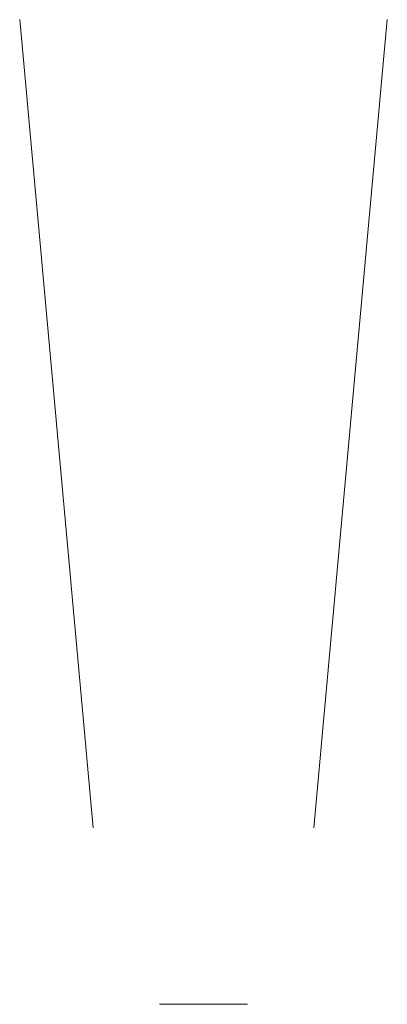
# Model space of a CAD drawing. Units: millimetres. Extents: x 345 to 395, y 449 to 583.
import ezdxf

# ---------------------------------------------------------------- set-up
doc = ezdxf.new("R2010")
doc.units = ezdxf.units.MM
doc.layers.add('M-CONS', color=8, linetype='Continuous', lineweight=13)

msp = doc.modelspace()

# ---------------------------------------------------------------- linework, layer by layer
at = {"layer": 'M-CONS'}
for p, q in [((345.41, 582.66, 10), (355.41, 472.66, 10)), ((395.41, 582.66, 10), (385.41, 472.66, 10)), ((364.41, 448.66, 10), (364.41, 448.66, 25)), ((364.41, 448.66, 10), (376.41, 448.66, 10)), ((376.41, 448.66, 10), (376.41, 448.66, 25))]:
    msp.add_line(p, q, dxfattribs=at)

doc.saveas('drawing.dxf')
